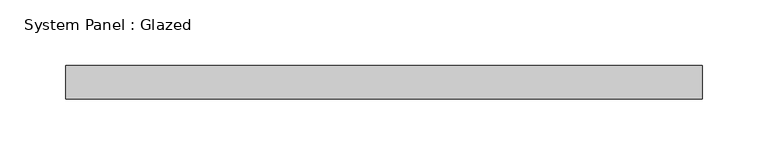
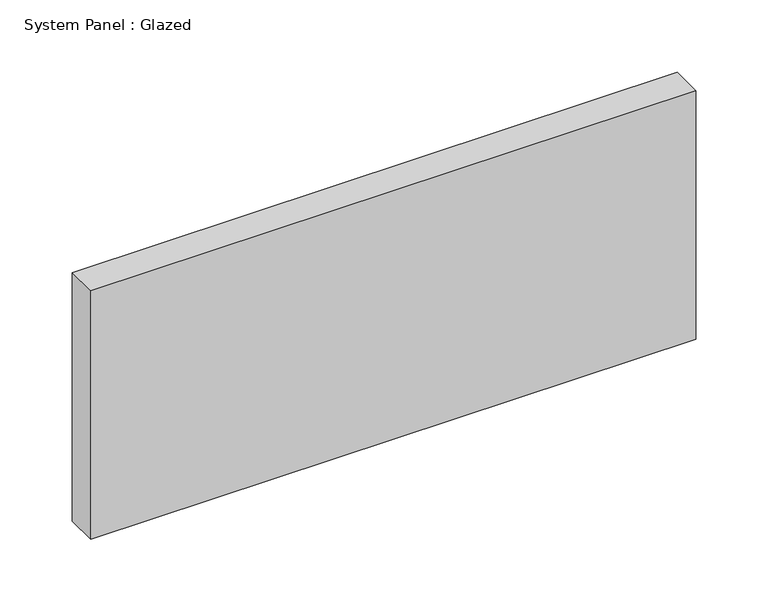
"""IFC4 building model written with IfcOpenShell, lengths in millimetres: plate geometry, System Panel : Glazed."""

from ifc_helpers import new_model, si_unit, origin, origin_with_axes, place, context, project, spatial, polyline, outline, extrude, source, transform, mapped, element, save


def system_panel_glazed_05e747e2(model_context):
    return source(origin(), model_context, "Body", "SweptSolid", [
        extrude(outline(polyline([(241.3, -44.45), (-241.3, -44.45), (-241.3, -19.05), (241.3, -19.05), (241.3, -44.45)])), origin_with_axes(), (0.0, 0.0, 1.0), 209.55),
    ])


if __name__ == "__main__":
    model = new_model("IFC4")
    model_context = context("Model", 3, world=origin())
    ifc_project = project(units=[si_unit("LENGTHUNIT", "METRE", prefix="MILLI")], contexts=[model_context])
    site = spatial("IfcSite", under=ifc_project)
    building = spatial("IfcBuilding", under=site)
    placement = place(None, origin())
    system_panel_glazed_shape = system_panel_glazed_05e747e2(model_context)
    element("IfcPlate", 1, ObjectType="System Panel : Glazed", at=placement, inside=building, context=model_context, shape_type="MappedRepresentation", body=[
        mapped(system_panel_glazed_shape, transform((0.0, 0.0, 0.0), x_axis=(1.0, 0.0, 0.0), y_axis=(0.0, 1.0, 0.0), z_axis=(0.0, 0.0, 1.0))),
    ])
    save(model, "model.ifc")

# Revit data of these elements
# Type "System Panel : Glazed"
#   Construction Type Id = "GSP4R"
#   Analytic Construction = "1/8 in Pilkington single glazing"
#   Visual Light Transmittance = 0.9
#   Solar Heat Gain Coefficient = 0.86
#   Heat Transfer Coefficient (U) = 1.18115 BTU/(h·ft²·°F)
#   Define Thermal Properties by = 1
# Element 1 (IfcPlate, "System Panel : Glazed")
#   Materials on its faces: "Glass"
# Materials
#   "Glass": class "Glass", colour RGB 0 128 192, transparency 0.75, Description = "Soda Lime Glass", Cost = 0
